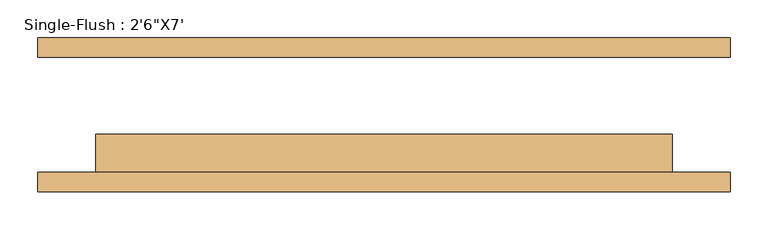
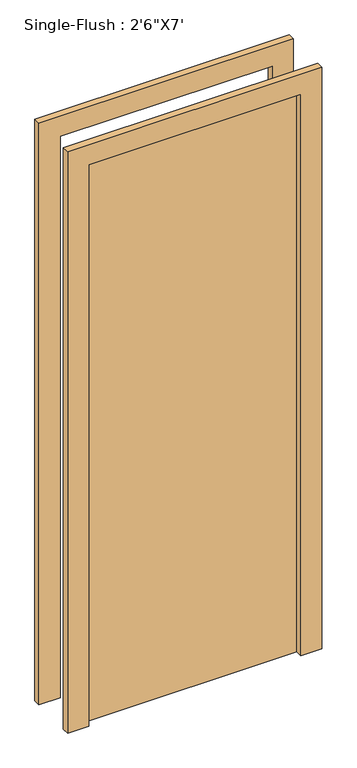
"""IFC4 building model written with IfcOpenShell, lengths in millimetres: door geometry."""

from ifc_helpers import new_model, si_unit, frame, origin, origin_with_axes, place, context, project, spatial, polyline, outline, extrude, source, transform, mapped, element, save


def door_e2b13fe9(model_context):
    return source(origin(), model_context, "Body", "SweptSolid", [
        extrude(outline(polyline([(2209.8, -457.2), (0.0, -457.2), (0.0, -381.0), (2133.6, -381.0), (2133.6, 381.0), (0.0, 381.0), (0.0, 457.2), (2209.8, 457.2), (2209.8, -457.2)])), frame((0.0, -101.6, 0.0), z_axis=(0.0, 1.0, 0.0), x_axis=(0.0, 0.0, 1.0)), (0.0, 0.0, 1.0), 25.4),
        extrude(outline(polyline([(2209.8, 457.2), (2209.8, -457.2), (0.0, -457.2), (0.0, -381.0), (2133.6, -381.0), (2133.6, 381.0), (0.0, 381.0), (0.0, 457.2), (2209.8, 457.2)])), frame((0.0, 76.2, 0.0), z_axis=(0.0, 1.0, 0.0), x_axis=(0.0, 0.0, 1.0)), (0.0, 0.0, 1.0), 25.4),
        extrude(outline(polyline([(381.0, -25.4), (381.0, -76.2), (-381.0, -76.2), (-381.0, -25.4), (381.0, -25.4)])), origin_with_axes(), (0.0, 0.0, 1.0), 2133.6),
    ])


if __name__ == "__main__":
    model = new_model("IFC4")
    model_context = context("Model", 3, world=origin())
    ifc_project = project(units=[si_unit("LENGTHUNIT", "METRE", prefix="MILLI")], contexts=[model_context])
    site = spatial("IfcSite", under=ifc_project)
    building = spatial("IfcBuilding", under=site)
    placement = place(None, origin())
    door_shape = door_e2b13fe9(model_context)
    element("IfcDoor", 1, ObjectType="Single-Flush : 2'6\"X7'", at=placement, inside=building, context=model_context, shape_type="MappedRepresentation", body=[
        mapped(door_shape, transform((0.0, 0.0, 0.0), x_axis=(1.0, 0.0, 0.0), y_axis=(0.0, 1.0, 0.0), z_axis=(0.0, 0.0, 1.0))),
    ])
    save(model, "model.ifc")

# Revit data of these elements
# Type "Single-Flush : 2'6\"X7'"
#   Type Mark = "10"
#   Construction Type Id = "MDOOR"
#   Assembly Code = "C1020"
#   Analytic Construction = "Metal"
#   Thickness = 0' - 2"
#   Heat Transfer Coefficient (U) = 0.651978 BTU/(h·ft²·°F)
#   Height = 7' - 0"
#   Trim Projection Ext = 0' - 1"
#   Trim Projection Int = 0' - 1"
#   Trim Width = 0' - 3"
#   Width = 2' - 6"
#   Define Thermal Properties by = 1
#   Door Material = Door - Panel
#   Frame Material = Door - Frame
#   Visual Light Transmittance = 0
#   Solar Heat Gain Coefficient = 0
#   Function = (empty or 0)
#   Wall Closure = (empty or 0)
# Element 1 (IfcDoor, "Single-Flush : 2'6\"X7'")
#   Materials on its faces: "Door - Frame", "Door - Panel"
# Materials
#   "Door - Panel": class "Wood", colour RGB 210 159 95, transparency 0, Cost = 0
#   "Door - Frame": colour RGB 118 70 51, transparency 0, Cost = 0
